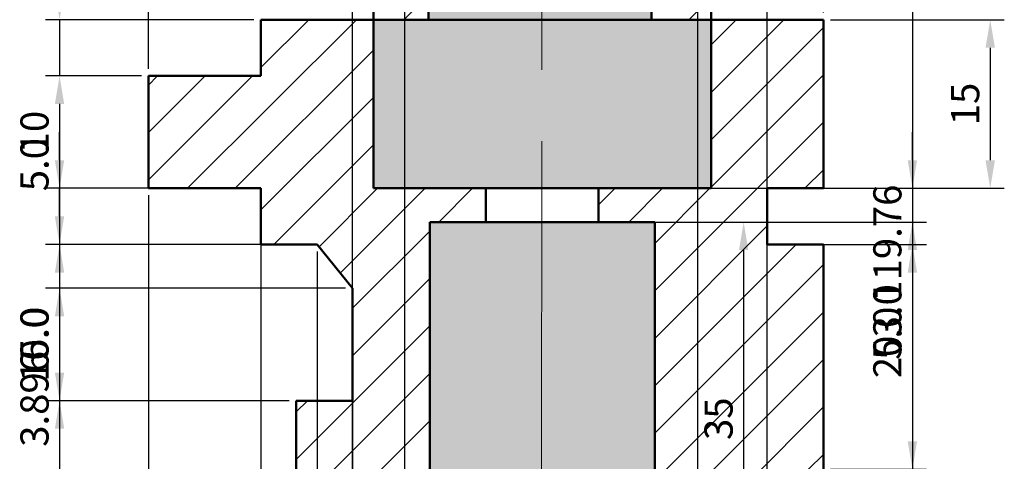
# Model space of a CAD drawing. Units: millimetres. Extents: x 1159 to 1466, y 1237 to 1440.
# Tile 5 of 6: x 1378 to 1466, y 1296 to 1336. Entities that reach past the tile are written whole.
import ezdxf

# ---------------------------------------------------------------- set-up
doc = ezdxf.new("R2010")
doc.units = ezdxf.units.MM
doc.linetypes.add('CENTER', pattern=[50.8, 31.75, -6.35, 6.35, -6.35])
for name, color, linetype, lineweight in [('M-CNTR', 1, 'CENTER', 18), ('M-DIMS', 2, 'Continuous', 25), ('M-HATC', 8, 'Continuous', 18), ('M-OUTL', 7, 'Continuous', 50)]:
    doc.layers.add(name, color=color, linetype=linetype, lineweight=lineweight)
doc.styles.get("Standard").update_dxf_attribs({"font": 'arial.ttf'})
doc.dimstyles.new('ISO-25', dxfattribs={"dimtxt": 2.5, "dimasz": 2.5, "dimexe": 1.25, "dimexo": 0.625, "dimtad": 1, "dimtxsty": 'Standard', "dimcen": 2.5, "dimadec": 0, "dimazin": 0, "dimtfac": 1, "dimtmove": 0, "dimatfit": 3, "dimfxl": 1, "dimarcsym": 0})

# ---------------------------------------------------------------- blocks, each defined once
blk = doc.blocks.new('*D22')
at = {"layer": 'Defpoints', "color": 0, "transparency": 16777216}
for p in [(1449.751, 1335.561), (1449.751, 1320.561), (1464.568, 1320.561)]:
    blk.add_point(p, dxfattribs=at)
at = {"layer": 'M-DIMS', "color": 0, "lineweight": -2, "transparency": 16777216}
for p, q in [((1450.376, 1335.561), (1465.818, 1335.561)), ((1464.568, 1333.061), (1464.568, 1323.061)), ((1450.376, 1320.561), (1465.818, 1320.561))]:
    blk.add_line(p, q, dxfattribs=at)
at = {"layer": 'M-DIMS', "color": 0, "transparency": 16777216}
for points in [[(1464.151, 1333.061), (1464.985, 1333.061), (1464.568, 1335.561)], [(1464.151, 1323.061), (1464.985, 1323.061), (1464.568, 1320.561)]]:
    blk.add_solid(points, dxfattribs=at)
at = {"layer": 'M-DIMS', "color": 0, "transparency": 16777216, "insert": (1462.667, 1328.061), "char_height": 2.5, "attachment_point": 5, "rotation": 90}
blk.add_mtext('15', dxfattribs=at)
blk = doc.blocks.new('*D42')
at = {"layer": 'Defpoints', "color": 0, "transparency": 16777216}
for p in [(1409.751, 1375.561), (1424.964, 1255.799), (1457.651, 1255.799)]:
    blk.add_point(p, dxfattribs=at)
at = {"layer": 'M-DIMS', "color": 0, "lineweight": -2, "transparency": 16777216}
for p, q in [((1410.376, 1375.561), (1458.901, 1375.561)), ((1457.651, 1373.061), (1457.651, 1258.299)), ((1425.589, 1255.799), (1458.901, 1255.799))]:
    blk.add_line(p, q, dxfattribs=at)
at = {"layer": 'M-DIMS', "color": 0, "transparency": 16777216}
for points in [[(1457.234, 1373.061), (1458.067, 1373.061), (1457.651, 1375.561)], [(1457.234, 1258.299), (1458.067, 1258.299), (1457.651, 1255.799)]]:
    blk.add_solid(points, dxfattribs=at)
at = {"layer": 'M-DIMS', "color": 0, "transparency": 16777216, "insert": (1455.749, 1315.68), "char_height": 2.5, "attachment_point": 5, "rotation": 90}
blk.add_mtext('119.76', dxfattribs=at)
blk = doc.blocks.new('*D43')
at = {"layer": 'Defpoints', "color": 0, "transparency": 16777216}
for p in [(1449.751, 1383.461), (1449.751, 1335.561), (1389.751, 1330.561)]:
    blk.add_point(p, dxfattribs=at)
at = {"layer": 'M-DIMS', "color": 0, "lineweight": -2, "transparency": 16777216}
for p, q in [((1389.751, 1331.186), (1389.751, 1384.711)), ((1449.751, 1336.186), (1449.751, 1384.711)), ((1392.251, 1383.461), (1447.251, 1383.461))]:
    blk.add_line(p, q, dxfattribs=at)
at = {"layer": 'M-DIMS', "color": 0, "transparency": 16777216}
for points in [[(1392.251, 1383.878), (1392.251, 1383.044), (1389.751, 1383.461)], [(1447.251, 1383.878), (1447.251, 1383.044), (1449.751, 1383.461)]]:
    blk.add_solid(points, dxfattribs=at)
at = {"layer": 'M-DIMS', "color": 0, "transparency": 16777216, "insert": (1419.751, 1385.362), "char_height": 2.5, "attachment_point": 5}
blk.add_mtext('60', dxfattribs=at)
blk = doc.blocks.new('*D44')
at = {"layer": 'Defpoints', "color": 0, "transparency": 16777216}
for p in [(1389.751, 1320.561), (1399.751, 1320.561), (1399.751, 1247.895)]:
    blk.add_point(p, dxfattribs=at)
at = {"layer": 'M-DIMS', "color": 0, "lineweight": -2, "transparency": 16777216}
for p, q in [((1389.751, 1319.936), (1389.751, 1246.645)), ((1399.751, 1319.936), (1399.751, 1246.645)), ((1392.251, 1247.895), (1397.251, 1247.895))]:
    blk.add_line(p, q, dxfattribs=at)
at = {"layer": 'M-DIMS', "color": 0, "transparency": 16777216}
for points in [[(1392.251, 1248.311), (1392.251, 1247.478), (1389.751, 1247.895)], [(1397.251, 1248.311), (1397.251, 1247.478), (1399.751, 1247.895)]]:
    blk.add_solid(points, dxfattribs=at)
at = {"layer": 'M-DIMS', "color": 0, "transparency": 16777216, "insert": (1394.751, 1249.796), "char_height": 2.5, "attachment_point": 5}
blk.add_mtext('10', dxfattribs=at)
blk = doc.blocks.new('*D45')
at = {"layer": 'Defpoints', "color": 0, "transparency": 16777216}
for p in [(1389.751, 1330.561), (1381.851, 1320.561), (1389.751, 1320.561)]:
    blk.add_point(p, dxfattribs=at)
at = {"layer": 'M-DIMS', "color": 0, "lineweight": -2, "transparency": 16777216}
for p, q in [((1389.126, 1330.561), (1380.601, 1330.561)), ((1381.851, 1328.061), (1381.851, 1323.061)), ((1389.126, 1320.561), (1380.601, 1320.561))]:
    blk.add_line(p, q, dxfattribs=at)
at = {"layer": 'M-DIMS', "color": 0, "transparency": 16777216}
for points in [[(1381.434, 1328.061), (1382.267, 1328.061), (1381.851, 1330.561)], [(1381.434, 1323.061), (1382.267, 1323.061), (1381.851, 1320.561)]]:
    blk.add_solid(points, dxfattribs=at)
at = {"layer": 'M-DIMS', "color": 0, "transparency": 16777216, "insert": (1379.949, 1325.561), "char_height": 2.5, "attachment_point": 5, "rotation": 90}
blk.add_mtext('10', dxfattribs=at)
blk = doc.blocks.new('*D47')
at = {"layer": 'Defpoints', "color": 0, "transparency": 16777216}
for p in [(1434.751, 1317.561), (1434.751, 1282.561), (1442.651, 1282.561)]:
    blk.add_point(p, dxfattribs=at)
at = {"layer": 'M-DIMS', "color": 0, "lineweight": -2, "transparency": 16777216}
for p, q in [((1435.376, 1317.561), (1443.901, 1317.561)), ((1442.651, 1315.061), (1442.651, 1285.061)), ((1435.376, 1282.561), (1443.901, 1282.561))]:
    blk.add_line(p, q, dxfattribs=at)
at = {"layer": 'M-DIMS', "color": 0, "transparency": 16777216}
for points in [[(1442.234, 1315.061), (1443.067, 1315.061), (1442.651, 1317.561)], [(1442.234, 1285.061), (1443.067, 1285.061), (1442.651, 1282.561)]]:
    blk.add_solid(points, dxfattribs=at)
at = {"layer": 'M-DIMS', "color": 0, "transparency": 16777216, "insert": (1440.749, 1300.061), "char_height": 2.5, "attachment_point": 5, "rotation": 90}
blk.add_mtext('35', dxfattribs=at)
blk = doc.blocks.new('*D50')
at = {"layer": 'Defpoints', "color": 0, "transparency": 16777216}
for p in [(1449.751, 1315.561), (1449.751, 1295.561), (1457.651, 1295.561)]:
    blk.add_point(p, dxfattribs=at)
at = {"layer": 'M-DIMS', "color": 0, "lineweight": -2, "transparency": 16777216}
for p, q in [((1450.376, 1315.561), (1458.901, 1315.561)), ((1457.651, 1313.061), (1457.651, 1298.061)), ((1450.376, 1295.561), (1458.901, 1295.561))]:
    blk.add_line(p, q, dxfattribs=at)
at = {"layer": 'M-DIMS', "color": 0, "transparency": 16777216}
for points in [[(1457.234, 1313.061), (1458.067, 1313.061), (1457.651, 1315.561)], [(1457.234, 1298.061), (1458.067, 1298.061), (1457.651, 1295.561)]]:
    blk.add_solid(points, dxfattribs=at)
at = {"layer": 'M-DIMS', "color": 0, "transparency": 16777216, "insert": (1455.749, 1305.561), "char_height": 2.5, "attachment_point": 5, "rotation": 90}
blk.add_mtext('20', dxfattribs=at)
blk = doc.blocks.new('*D51')
at = {"layer": 'Defpoints', "color": 0, "transparency": 16777216}
for p in [(1402.885, 1301.665), (1381.851, 1281.665), (1402.885, 1281.665)]:
    blk.add_point(p, dxfattribs=at)
at = {"layer": 'M-DIMS', "color": 0, "lineweight": -2, "transparency": 16777216}
for p, q in [((1402.26, 1301.665), (1380.601, 1301.665)), ((1381.851, 1299.165), (1381.851, 1284.165)), ((1402.26, 1281.665), (1380.601, 1281.665))]:
    blk.add_line(p, q, dxfattribs=at)
at = {"layer": 'M-DIMS', "color": 0, "transparency": 16777216}
for points in [[(1381.434, 1299.165), (1382.267, 1299.165), (1381.851, 1301.665)], [(1381.434, 1284.165), (1382.267, 1284.165), (1381.851, 1281.665)]]:
    blk.add_solid(points, dxfattribs=at)
at = {"layer": 'M-DIMS', "color": 0, "transparency": 16777216, "insert": (1379.949, 1291.665), "char_height": 2.5, "attachment_point": 5, "rotation": 90}
blk.add_mtext('20', dxfattribs=at)
blk = doc.blocks.new('*D58')
at = {"layer": 'Defpoints', "color": 0, "transparency": 16777216}
for p in [(1399.751, 1335.561), (1381.851, 1330.561), (1389.751, 1330.561)]:
    blk.add_point(p, dxfattribs=at)
at = {"layer": 'M-DIMS', "color": 0, "lineweight": -2, "transparency": 16777216}
for p, q in [((1381.851, 1338.061), (1381.851, 1340.561)), ((1399.126, 1335.561), (1380.601, 1335.561)), ((1381.851, 1335.561), (1381.851, 1330.561)), ((1389.126, 1330.561), (1380.601, 1330.561)), ((1381.851, 1328.061), (1381.851, 1319.768))]:
    blk.add_line(p, q, dxfattribs=at)
at = {"layer": 'M-DIMS', "color": 0, "transparency": 16777216}
for points in [[(1381.434, 1338.061), (1382.267, 1338.061), (1381.851, 1335.561)], [(1381.434, 1328.061), (1382.267, 1328.061), (1381.851, 1330.561)]]:
    blk.add_solid(points, dxfattribs=at)
at = {"layer": 'M-DIMS', "color": 0, "transparency": 16777216, "insert": (1379.949, 1322.665), "char_height": 2.5, "attachment_point": 5, "rotation": 90}
blk.add_mtext('5.0', dxfattribs=at)
blk = doc.blocks.new('*D59')
at = {"layer": 'Defpoints', "color": 0, "transparency": 16777216}
for p in [(1419.751, 1320.561), (1419.751, 1317.561), (1457.651, 1317.561)]:
    blk.add_point(p, dxfattribs=at)
at = {"layer": 'M-DIMS', "color": 0, "lineweight": -2, "transparency": 16777216}
for p, q in [((1457.651, 1323.061), (1457.651, 1325.561)), ((1420.376, 1320.561), (1458.901, 1320.561)), ((1457.651, 1320.561), (1457.651, 1317.561)), ((1420.376, 1317.561), (1458.901, 1317.561)), ((1457.651, 1315.061), (1457.651, 1306.77))]:
    blk.add_line(p, q, dxfattribs=at)
at = {"layer": 'M-DIMS', "color": 0, "transparency": 16777216}
for points in [[(1457.234, 1323.061), (1458.067, 1323.061), (1457.651, 1320.561)], [(1457.234, 1315.061), (1458.067, 1315.061), (1457.651, 1317.561)]]:
    blk.add_solid(points, dxfattribs=at)
at = {"layer": 'M-DIMS', "color": 0, "transparency": 16777216, "insert": (1455.749, 1309.665), "char_height": 2.5, "attachment_point": 5, "rotation": 90}
blk.add_mtext('3.0', dxfattribs=at)
blk = doc.blocks.new('*D60')
at = {"layer": 'Defpoints', "color": 0, "transparency": 16777216}
for p in [(1444.751, 1320.561), (1444.751, 1315.561), (1457.651, 1315.561)]:
    blk.add_point(p, dxfattribs=at)
at = {"layer": 'M-DIMS', "color": 0, "lineweight": -2, "transparency": 16777216}
for p, q in [((1457.651, 1323.061), (1457.651, 1325.561)), ((1445.376, 1320.561), (1458.901, 1320.561)), ((1457.651, 1320.561), (1457.651, 1315.561)), ((1445.376, 1315.561), (1458.901, 1315.561)), ((1457.651, 1313.061), (1457.651, 1304.768))]:
    blk.add_line(p, q, dxfattribs=at)
at = {"layer": 'M-DIMS', "color": 0, "transparency": 16777216}
for points in [[(1457.234, 1323.061), (1458.067, 1323.061), (1457.651, 1320.561)], [(1457.234, 1313.061), (1458.067, 1313.061), (1457.651, 1315.561)]]:
    blk.add_solid(points, dxfattribs=at)
at = {"layer": 'M-DIMS', "color": 0, "transparency": 16777216, "insert": (1455.749, 1307.665), "char_height": 2.5, "attachment_point": 5, "rotation": 90}
blk.add_mtext('5.0', dxfattribs=at)
blk = doc.blocks.new('*D62')
at = {"layer": 'Defpoints', "color": 0, "transparency": 16777216}
for p in [(1399.751, 1320.561), (1381.851, 1315.561), (1404.751, 1315.561)]:
    blk.add_point(p, dxfattribs=at)
at = {"layer": 'M-DIMS', "color": 0, "lineweight": -2, "transparency": 16777216}
for p, q in [((1381.851, 1323.061), (1381.851, 1325.561)), ((1399.126, 1320.561), (1380.601, 1320.561)), ((1381.851, 1320.561), (1381.851, 1315.561)), ((1404.126, 1315.561), (1380.601, 1315.561)), ((1381.851, 1313.061), (1381.851, 1304.768))]:
    blk.add_line(p, q, dxfattribs=at)
at = {"layer": 'M-DIMS', "color": 0, "transparency": 16777216}
for points in [[(1381.434, 1323.061), (1382.267, 1323.061), (1381.851, 1320.561)], [(1381.434, 1313.061), (1382.267, 1313.061), (1381.851, 1315.561)]]:
    blk.add_solid(points, dxfattribs=at)
at = {"layer": 'M-DIMS', "color": 0, "transparency": 16777216, "insert": (1379.949, 1307.665), "char_height": 2.5, "attachment_point": 5, "rotation": 90}
blk.add_mtext('5.0', dxfattribs=at)
blk = doc.blocks.new('*D63')
at = {"layer": 'Defpoints', "color": 0, "transparency": 16777216}
for p in [(1404.751, 1315.561), (1381.851, 1311.665), (1407.885, 1311.665)]:
    blk.add_point(p, dxfattribs=at)
at = {"layer": 'M-DIMS', "color": 0, "lineweight": -2, "transparency": 16777216}
for p, q in [((1381.851, 1318.061), (1381.851, 1320.561)), ((1404.126, 1315.561), (1380.601, 1315.561)), ((1381.851, 1315.561), (1381.851, 1311.665)), ((1407.26, 1311.665), (1380.601, 1311.665)), ((1381.851, 1309.165), (1381.851, 1296.982))]:
    blk.add_line(p, q, dxfattribs=at)
at = {"layer": 'M-DIMS', "color": 0, "transparency": 16777216}
for points in [[(1381.434, 1318.061), (1382.267, 1318.061), (1381.851, 1315.561)], [(1381.434, 1309.165), (1382.267, 1309.165), (1381.851, 1311.665)]]:
    blk.add_solid(points, dxfattribs=at)
at = {"layer": 'M-DIMS', "color": 0, "transparency": 16777216, "insert": (1379.949, 1301.824), "char_height": 2.5, "attachment_point": 5, "rotation": 90}
blk.add_mtext('3.896', dxfattribs=at)
blk = doc.blocks.new('*D64')
at = {"layer": 'Defpoints', "color": 0, "transparency": 16777216}
for p in [(1407.885, 1311.665), (1381.851, 1301.665), (1402.885, 1301.665)]:
    blk.add_point(p, dxfattribs=at)
at = {"layer": 'M-DIMS', "color": 0, "lineweight": -2, "transparency": 16777216}
for p, q in [((1407.26, 1311.665), (1380.601, 1311.665)), ((1381.851, 1309.165), (1381.851, 1304.165)), ((1402.26, 1301.665), (1380.601, 1301.665))]:
    blk.add_line(p, q, dxfattribs=at)
at = {"layer": 'M-DIMS', "color": 0, "transparency": 16777216}
for points in [[(1381.434, 1309.165), (1382.267, 1309.165), (1381.851, 1311.665)], [(1381.434, 1304.165), (1382.267, 1304.165), (1381.851, 1301.665)]]:
    blk.add_solid(points, dxfattribs=at)
at = {"layer": 'M-DIMS', "color": 0, "transparency": 16777216, "insert": (1379.949, 1306.665), "char_height": 2.5, "attachment_point": 5, "rotation": 90}
blk.add_mtext('10.0', dxfattribs=at)
blk = doc.blocks.new('*D65')
at = {"layer": 'Defpoints', "color": 0, "transparency": 16777216}
for p in [(1399.751, 1315.561), (1402.885, 1301.665), (1402.885, 1247.895)]:
    blk.add_point(p, dxfattribs=at)
at = {"layer": 'M-DIMS', "color": 0, "lineweight": -2, "transparency": 16777216}
for p, q in [((1399.751, 1314.936), (1399.751, 1246.645)), ((1402.885, 1301.04), (1402.885, 1246.645)), ((1397.251, 1247.895), (1394.751, 1247.895)), ((1399.751, 1247.895), (1402.885, 1247.895)), ((1405.385, 1247.895), (1417.559, 1247.895))]:
    blk.add_line(p, q, dxfattribs=at)
at = {"layer": 'M-DIMS', "color": 0, "transparency": 16777216}
for points in [[(1397.251, 1248.311), (1397.251, 1247.478), (1399.751, 1247.895)], [(1405.385, 1248.311), (1405.385, 1247.478), (1402.885, 1247.895)]]:
    blk.add_solid(points, dxfattribs=at)
at = {"layer": 'M-DIMS', "color": 0, "transparency": 16777216, "insert": (1412.722, 1249.797), "char_height": 2.5, "attachment_point": 5}
blk.add_mtext('3.134', dxfattribs=at)
blk = doc.blocks.new('*D66')
at = {"layer": 'Defpoints', "color": 0, "transparency": 16777216}
for p in [(1404.751, 1315.561), (1402.885, 1301.665), (1404.751, 1247.895)]:
    blk.add_point(p, dxfattribs=at)
at = {"layer": 'M-DIMS', "color": 0, "lineweight": -2, "transparency": 16777216}
for p, q in [((1404.751, 1314.936), (1404.751, 1246.645)), ((1402.885, 1301.04), (1402.885, 1246.645)), ((1400.385, 1247.895), (1397.885, 1247.895)), ((1402.885, 1247.895), (1404.751, 1247.895)), ((1407.251, 1247.895), (1419.2, 1247.895))]:
    blk.add_line(p, q, dxfattribs=at)
at = {"layer": 'M-DIMS', "color": 0, "transparency": 16777216}
for points in [[(1400.385, 1248.311), (1400.385, 1247.478), (1402.885, 1247.895)], [(1407.251, 1248.311), (1407.251, 1247.478), (1404.751, 1247.895)]]:
    blk.add_solid(points, dxfattribs=at)
at = {"layer": 'M-DIMS', "color": 0, "transparency": 16777216, "insert": (1414.475, 1249.796), "char_height": 2.5, "attachment_point": 5}
blk.add_mtext('1.866', dxfattribs=at)
blk = doc.blocks.new('*D67')
at = {"layer": 'Defpoints', "color": 0, "transparency": 16777216}
for p in [(1404.751, 1315.561), (1407.885, 1311.665), (1407.885, 1247.895)]:
    blk.add_point(p, dxfattribs=at)
at = {"layer": 'M-DIMS', "color": 0, "lineweight": -2, "transparency": 16777216}
for p, q in [((1404.751, 1314.936), (1404.751, 1246.645)), ((1407.885, 1311.04), (1407.885, 1246.645)), ((1402.251, 1247.895), (1399.751, 1247.895)), ((1404.751, 1247.895), (1407.885, 1247.895)), ((1410.385, 1247.895), (1422.559, 1247.895))]:
    blk.add_line(p, q, dxfattribs=at)
at = {"layer": 'M-DIMS', "color": 0, "transparency": 16777216}
for points in [[(1402.251, 1248.311), (1402.251, 1247.478), (1404.751, 1247.895)], [(1410.385, 1248.311), (1410.385, 1247.478), (1407.885, 1247.895)]]:
    blk.add_solid(points, dxfattribs=at)
at = {"layer": 'M-DIMS', "color": 0, "transparency": 16777216, "insert": (1417.722, 1249.797), "char_height": 2.5, "attachment_point": 5}
blk.add_mtext('3.134', dxfattribs=at)
blk = doc.blocks.new('*D74')
at = {"layer": 'Defpoints', "color": 0, "transparency": 16777216}
for p in [(1412.534, 1383.461), (1407.885, 1271.665), (1412.534, 1264.983)]:
    blk.add_point(p, dxfattribs=at)
at = {"layer": 'M-DIMS', "color": 0, "lineweight": -2, "transparency": 16777216}
for p, q in [((1407.885, 1272.29), (1407.885, 1384.711)), ((1412.534, 1265.608), (1412.534, 1384.711)), ((1405.385, 1383.461), (1402.885, 1383.461)), ((1407.885, 1383.461), (1412.534, 1383.461)), ((1415.034, 1383.461), (1427.326, 1383.461))]:
    blk.add_line(p, q, dxfattribs=at)
at = {"layer": 'M-DIMS', "color": 0, "transparency": 16777216}
for points in [[(1405.385, 1383.878), (1405.385, 1383.044), (1407.885, 1383.461)], [(1415.034, 1383.878), (1415.034, 1383.044), (1412.534, 1383.461)]]:
    blk.add_solid(points, dxfattribs=at)
at = {"layer": 'M-DIMS', "color": 0, "transparency": 16777216, "insert": (1422.43, 1385.362), "char_height": 2.5, "attachment_point": 5}
blk.add_mtext('4.649', dxfattribs=at)
blk = doc.blocks.new('*D75')
at = {"layer": 'Defpoints', "color": 0, "transparency": 16777216}
for p in [(1444.751, 1383.461), (1444.751, 1270.561), (1438.586, 1264.983)]:
    blk.add_point(p, dxfattribs=at)
at = {"layer": 'M-DIMS', "color": 0, "lineweight": -2, "transparency": 16777216}
for p, q in [((1438.586, 1265.608), (1438.586, 1384.711)), ((1444.751, 1271.186), (1444.751, 1384.711)), ((1436.086, 1383.461), (1433.586, 1383.461)), ((1438.586, 1383.461), (1444.751, 1383.461)), ((1447.251, 1383.461), (1459.469, 1383.461))]:
    blk.add_line(p, q, dxfattribs=at)
at = {"layer": 'M-DIMS', "color": 0, "transparency": 16777216}
for points in [[(1436.086, 1383.878), (1436.086, 1383.044), (1438.586, 1383.461)], [(1447.251, 1383.878), (1447.251, 1383.044), (1444.751, 1383.461)]]:
    blk.add_solid(points, dxfattribs=at)
at = {"layer": 'M-DIMS', "color": 0, "transparency": 16777216, "insert": (1454.61, 1385.362), "char_height": 2.5, "attachment_point": 5}
blk.add_mtext('6.165', dxfattribs=at)

msp = doc.modelspace()

# ---------------------------------------------------------------- hatches: boundary and pattern name
at = {"layer": 'M-HATC'}
h = msp.add_hatch(dxfattribs=at)
h.set_pattern_fill('ANSI31', color=256, scale=0.94)
h.set_pattern_definition([(45, (0, -76.8912), (-2.11036, 2.11036), [])])
h.paths.add_polyline_path([(1414.6374, 1375.561), (1409.7508, 1375.561), (1409.7508, 1335.561), (1414.6374, 1335.561)])
h.paths.add_polyline_path([(1439.7508, 1375.561), (1434.4515, 1375.561), (1434.4515, 1335.561), (1439.7508, 1335.561)])
h.paths.add_polyline_path([(1449.7508, 1315.561), (1444.7508, 1315.561), (1444.7508, 1320.561), (1449.7508, 1320.561), (1449.7508, 1335.561), (1439.7508, 1335.561), (1439.7508, 1320.561), (1429.7508, 1320.561), (1429.7508, 1317.561), (1434.7508, 1317.561), (1434.7508, 1282.561), (1429.7508, 1282.561), (1429.7508, 1267.561, -0.1562704), (1427.7989, 1264.9827), (1438.5857, 1264.9827), (1444.7508, 1270.561), (1444.7508, 1275.561), (1444.7508, 1295.561), (1449.7508, 1295.561)])
h.paths.add_polyline_path([(1414.7508, 1317.561), (1419.7508, 1317.561), (1419.7508, 1320.561), (1409.7508, 1320.561), (1409.7508, 1335.561), (1399.7508, 1335.561), (1399.7508, 1330.561), (1389.7508, 1330.561), (1389.7508, 1320.561), (1399.7508, 1320.561), (1399.7508, 1315.561), (1404.7508, 1315.561), (1407.8849, 1311.6652), (1407.8849, 1301.6652), (1402.8849, 1301.6652), (1402.8849, 1281.6652), (1407.8849, 1281.6652), (1407.8849, 1271.6652), (1412.5343, 1264.9827), (1421.7027, 1264.9827, -0.1562704), (1419.7508, 1267.561), (1419.7508, 1282.561), (1414.7508, 1282.561)])
h.paths.add_polyline_path([(1424.6651, 1264.0191, -0.1502665), (1421.7027, 1264.9827), (1412.5343, 1264.9827), (1415.9205, 1260.1158, 0.2337513), (1424.6588, 1255.7945)])
h.paths.add_polyline_path([(1433.7538, 1260.6108), (1438.5857, 1264.9827), (1427.7989, 1264.9827, -0.1585441), (1424.6651, 1264.0191), (1424.6588, 1255.7945, 0.248431)])
h = msp.add_hatch(color=256, dxfattribs=at)
h.set_gradient(color1=(34, 52, 110), color2=(0, 0, 0))
h.paths.add_polyline_path([(1424.7508, 1375.561), (1414.6374, 1375.561), (1414.6374, 1335.561), (1424.7201, 1335.561)])
h.paths.add_polyline_path([(1434.4515, 1375.561), (1424.7508, 1375.561), (1424.7201, 1335.561), (1434.4515, 1335.561)])
h.paths.add_polyline_path([(1424.7201, 1335.561), (1414.6374, 1335.561), (1409.7508, 1335.561), (1409.7508, 1320.561), (1424.7085, 1320.561)])
h.paths.add_polyline_path([(1439.7508, 1335.561), (1424.7201, 1335.561), (1424.7085, 1320.561), (1424.7508, 1320.561), (1439.7508, 1320.561)])
h.paths.add_polyline_path([(1434.7508, 1317.561), (1429.7508, 1317.561), (1424.7062, 1317.561), (1424.6793, 1282.561), (1424.7508, 1282.561), (1434.7508, 1282.561)])
h.paths.add_polyline_path([(1424.7062, 1317.561), (1419.7508, 1317.561), (1414.7508, 1317.561), (1414.7508, 1282.561), (1424.6793, 1282.561)])
h.paths.add_polyline_path([(1424.6793, 1282.561), (1419.7508, 1282.561), (1419.7508, 1267.561), (1424.6678, 1267.561)])
h.paths.add_polyline_path([(1429.7508, 1282.561), (1424.6793, 1282.561), (1424.6678, 1267.561), (1429.7508, 1267.561)])
h.paths.add_polyline_path([(1424.6678, 1267.561), (1419.7508, 1267.561, 0.2389901), (1424.6658, 1264.9833)])
h.paths.add_polyline_path([(1429.7508, 1267.561), (1424.6678, 1267.561), (1424.6658, 1264.9833, 0.2463189)])
h.paths.add_polyline_path([(1419.7508, 1267.561, 0.1562704), (1421.7027, 1264.9827), (1424.7508, 1264.9827, -0.2426514)])
h.paths.add_polyline_path([(1429.7508, 1267.561, -0.2426514), (1424.7508, 1264.9827), (1427.7989, 1264.9827, 0.1562704)], flags=17)
h.paths.add_polyline_path([(1427.7989, 1264.9827), (1424.7508, 1264.9827), (1424.6658, 1264.9827), (1424.6651, 1264.0191, 0.1585441)])
h.paths.add_polyline_path([(1424.6658, 1264.9827), (1421.7027, 1264.9827, 0.1502665), (1424.6651, 1264.0191)])

# ---------------------------------------------------------------- linework, layer by layer
at = {"layer": 'M-CNTR'}
msp.add_line((1424.7508, 1375.561), (1424.6588, 1255.7945), dxfattribs=at)
at = {"layer": 'M-OUTL'}
for p, q in [((1409.7508, 1335.561), (1409.7508, 1375.561)), ((1414.6374, 1335.561), (1414.6374, 1375.561)), ((1434.4515, 1375.561), (1434.4515, 1335.561)), ((1439.7508, 1375.561), (1439.7508, 1335.561)), ((1409.7508, 1335.561), (1399.7508, 1335.561)), ((1399.7508, 1335.561), (1399.7508, 1330.561)), ((1439.7508, 1335.561), (1409.7508, 1335.561)), ((1409.7508, 1335.561), (1409.7508, 1320.561)), ((1439.7508, 1335.561), (1449.7508, 1335.561)), ((1439.7508, 1320.561), (1439.7508, 1335.561)), ((1449.7508, 1335.561), (1449.7508, 1320.561)), ((1399.7508, 1330.561), (1389.7508, 1330.561)), ((1389.7508, 1330.561), (1389.7508, 1320.561)), ((1389.7508, 1320.561), (1399.7508, 1320.561)), ((1399.7508, 1320.561), (1399.7508, 1315.561)), ((1409.7508, 1320.561), (1439.7508, 1320.561)), ((1424.7508, 1320.561), (1419.7508, 1320.561)), ((1419.7508, 1320.561), (1419.7508, 1317.561)), ((1429.7508, 1317.561), (1429.7508, 1320.561)), ((1449.7508, 1320.561), (1444.7508, 1320.561)), ((1444.7508, 1320.561), (1444.7508, 1315.561)), ((1419.7508, 1317.561), (1414.7508, 1317.561)), ((1414.7508, 1317.561), (1414.7508, 1282.561)), ((1419.7508, 1317.561), (1429.7508, 1317.561)), ((1434.7508, 1317.561), (1429.7508, 1317.561)), ((1434.7508, 1282.561), (1434.7508, 1317.561)), ((1399.7508, 1315.561), (1404.7508, 1315.561)), ((1404.7508, 1315.561), (1407.8849, 1311.6652)), ((1444.7508, 1315.561), (1449.7508, 1315.561)), ((1449.7508, 1315.561), (1449.7508, 1295.561)), ((1407.8849, 1311.6652), (1407.8849, 1301.6652)), ((1407.8849, 1301.6652), (1402.8849, 1301.6652)), ((1402.8849, 1301.6652), (1402.8849, 1281.6652))]:
    msp.add_line(p, q, dxfattribs=at)

# ---------------------------------------------------------------- dimensions: what is measured, and where the dimension line sits
at = {"layer": 'M-DIMS'}
for base, p1, p2, override, picture, middle in [((1449.7508, 1383.461), (1389.7508, 1330.561), (1449.7508, 1335.561), {"dimdec": 0, "dimlfac": 1, "dimrnd": 0, "dimzin": 0, "dimdsep": 46, "dimlunit": 2}, '*D43', (1419.7508, 1385.3624)), ((1412.5343, 1383.461), (1407.8849, 1271.6652), (1412.5343, 1264.9827), {"dimdec": 3, "dimlfac": 1, "dimrnd": 0, "dimzin": 0, "dimdsep": 46, "dimlunit": 2}, '*D74', (1422.4303, 1385.3624)), ((1444.7508, 1383.461), (1438.5857, 1264.9827), (1444.7508, 1270.561), {"dimdec": 3, "dimlfac": 1, "dimrnd": 0, "dimzin": 0, "dimdsep": 46, "dimlunit": 2}, '*D75', (1454.6101, 1385.3624)), ((1399.7508, 1247.8945), (1389.7508, 1320.561), (1399.7508, 1320.561), {"dimdec": 0, "dimlfac": 1, "dimrnd": 0, "dimzin": 0, "dimdsep": 46, "dimlunit": 2}, '*D44', (1394.7508, 1249.796)), ((1402.8849, 1247.8945), (1399.7508, 1315.561), (1402.8849, 1301.6652), {"dimdec": 3, "dimlfac": 1, "dimrnd": 0, "dimzin": 0, "dimdsep": 46, "dimlunit": 2}, '*D65', (1412.722, 1249.7968)), ((1404.7508, 1247.8945), (1402.8849, 1301.6652), (1404.7508, 1315.561), {"dimdec": 3, "dimlfac": 1, "dimrnd": 0, "dimzin": 0, "dimdsep": 46, "dimlunit": 2}, '*D66', (1414.4754, 1249.796)), ((1407.8849, 1247.8945), (1404.7508, 1315.561), (1407.8849, 1311.6652), {"dimdec": 3, "dimlfac": 1, "dimrnd": 0, "dimzin": 0, "dimdsep": 46, "dimlunit": 2}, '*D67', (1417.722, 1249.7968))]:
    dim = msp.add_linear_dim(base=base, p1=p1, p2=p2, dimstyle='ISO-25', override=override, dxfattribs=at)
    dim.commit()
    dim.dimension.update_dxf_attribs({"geometry": picture, "text_midpoint": middle})
for base, p1, p2, angle, override, picture, middle in [((1457.6508, 1255.7988), (1409.7508, 1375.561), (1424.9638, 1255.7988), 90, {"dimdec": 2, "dimlfac": 1, "dimrnd": 0, "dimzin": 0, "dimdsep": 46, "dimlunit": 2}, '*D42', (1455.7494, 1315.6799)), ((1381.8508, 1330.561), (1399.7508, 1335.561), (1389.7508, 1330.561), 90, {"dimdec": 1, "dimlfac": 1, "dimrnd": 0, "dimzin": 0, "dimdsep": 46, "dimlunit": 2}, '*D58', (1379.9494, 1322.6645)), ((1464.5682, 1320.561), (1449.7508, 1335.561), (1449.7508, 1320.561), 90, {"dimclrd": 0, "dimclre": 0, "dimclrt": 0}, '*D22', (1462.6667, 1328.061)), ((1381.8508, 1320.561), (1389.7508, 1330.561), (1389.7508, 1320.561), 90, {"dimdec": 0, "dimlfac": 1, "dimrnd": 0, "dimzin": 0, "dimdsep": 46, "dimlunit": 2}, '*D45', (1379.9494, 1325.561)), ((1381.8508, 1315.561), (1399.7508, 1320.561), (1404.7508, 1315.561), 90, {"dimdec": 1, "dimlfac": 1, "dimrnd": 0, "dimzin": 0, "dimdsep": 46, "dimlunit": 2}, '*D62', (1379.9494, 1307.6645)), ((1457.6508, 1317.561), (1419.7508, 1320.561), (1419.7508, 1317.561), 90, {"dimdec": 1, "dimlfac": 1, "dimrnd": 0, "dimzin": 0, "dimdsep": 46, "dimlunit": 2}, '*D59', (1455.7485, 1309.6654)), ((1457.6508, 1315.561), (1444.7508, 1320.561), (1444.7508, 1315.561), 90, {"dimdec": 1, "dimlfac": 1, "dimrnd": 0, "dimzin": 0, "dimdsep": 46, "dimlunit": 2}, '*D60', (1455.7494, 1307.6645)), ((1381.8508, 1311.6652), (1404.7508, 1315.561), (1407.8849, 1311.6652), 90, {"dimdec": 3, "dimlfac": 1, "dimrnd": 0, "dimzin": 0, "dimdsep": 46, "dimlunit": 2}, '*D63', (1379.9485, 1301.8238)), ((1442.6508, 1282.561), (1434.7508, 1317.561), (1434.7508, 1282.561), 270, {"dimdec": 0, "dimlfac": 1, "dimrnd": 0, "dimzin": 0, "dimdsep": 46, "dimlunit": 2}, '*D47', (1440.7485, 1300.061)), ((1457.6508, 1295.561), (1449.7508, 1315.561), (1449.7508, 1295.561), 270, {"dimdec": 0, "dimlfac": 1, "dimrnd": 0, "dimzin": 0, "dimdsep": 46, "dimlunit": 2}, '*D50', (1455.7494, 1305.561)), ((1381.8508, 1301.6652), (1407.8849, 1311.6652), (1402.8849, 1301.6652), 90, {"dimdec": 1, "dimlfac": 1, "dimrnd": 0, "dimzin": 0, "dimdsep": 46, "dimlunit": 2}, '*D64', (1379.9494, 1306.6652)), ((1381.8508, 1281.6652), (1402.8849, 1301.6652), (1402.8849, 1281.6652), 90, {"dimdec": 0, "dimlfac": 1, "dimrnd": 0, "dimzin": 0, "dimdsep": 46, "dimlunit": 2}, '*D51', (1379.9494, 1291.6652))]:
    dim = msp.add_linear_dim(base=base, p1=p1, p2=p2, angle=angle, dimstyle='ISO-25', override=override, dxfattribs=at)
    dim.commit()
    dim.dimension.update_dxf_attribs({"geometry": picture, "text_midpoint": middle})

doc.saveas('drawing.dxf')
